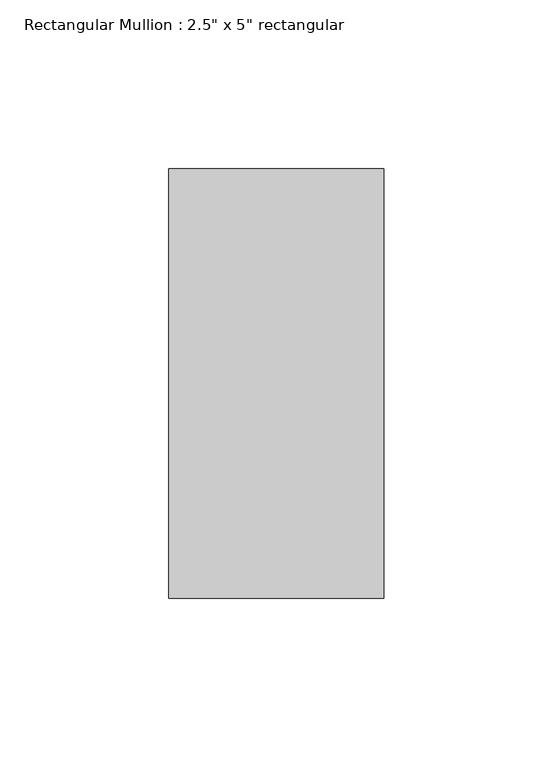
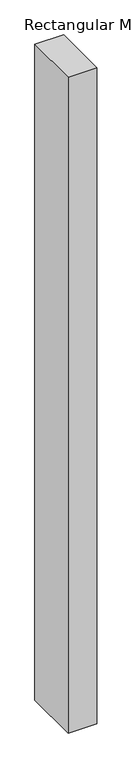
"""IFC4 building model written with IfcOpenShell, lengths in millimetres: member geometry."""

from ifc_helpers import new_model, si_unit, frame, origin, place, context, project, spatial, polyline, outline, extrude, source, transform, mapped, element, save


def member_f3ef6fbd(model_context):
    return source(origin(), model_context, "Body", "SweptSolid", [
        extrude(outline(polyline([(0.0, 63.5), (0.0, -63.5), (-63.5, -63.5), (-63.5, 63.5), (0.0, 63.5)])), frame((0.0, 0.0, -1535.0629342), z_axis=(0.0, 0.0, 1.0), x_axis=(1.0, 0.0, 0.0)), (0.0, 0.0, 1.0), 1535.0629342),
    ])


if __name__ == "__main__":
    model = new_model("IFC4")
    model_context = context("Model", 3, world=origin())
    ifc_project = project(units=[si_unit("LENGTHUNIT", "METRE", prefix="MILLI")], contexts=[model_context])
    site = spatial("IfcSite", under=ifc_project)
    building = spatial("IfcBuilding", under=site)
    placement = place(None, origin())
    member_shape = member_f3ef6fbd(model_context)
    element("IfcMember", 1, ObjectType="Rectangular Mullion : 2.5\" x 5\" rectangular", at=placement, inside=building, context=model_context, shape_type="MappedRepresentation", body=[
        mapped(member_shape, transform((0.0, 0.0, 0.0), x_axis=(1.0, 0.0, 0.0), y_axis=(0.0, 1.0, 0.0), z_axis=(0.0, 0.0, 1.0))),
    ])
    save(model, "model.ifc")

# Revit data of these elements
# Type "Rectangular Mullion : 2.5\" x 5\" rectangular"
#   built-in parameter 1007304 = 0.416667 (stored number, unit not read)
#   built-in parameter 1007301 = 0.104167 (stored number, unit not read)
#   built-in parameter 1007300 = 0.104167 (stored number, unit not read)
# Element 1 (IfcMember, "Rectangular Mullion : 2.5\" x 5\" rectangular")
#   Materials on its faces: "Aluminum"
# Materials
#   "Aluminum": class "Metal", colour RGB 247 247 247, transparency 0, Description = "Aluminum 6061", Cost = 0
